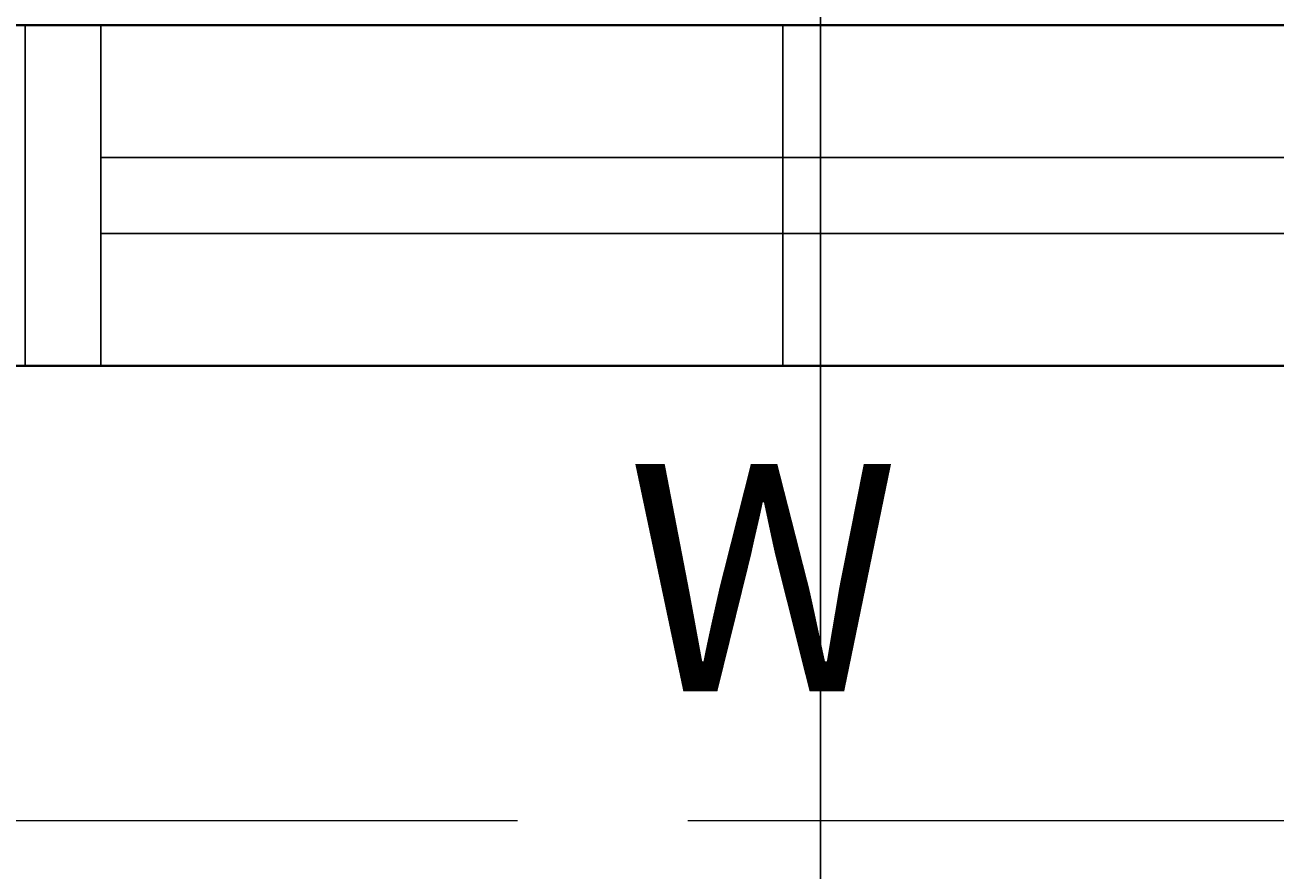
# Model space of a CAD drawing. Units: inches. Extents: x -301 to 715, y -607 to 364.
# Tile 59 of 141: x -144 to -111, y -237 to -215. Entities that reach past the tile are written whole.
import ezdxf

# ---------------------------------------------------------------- set-up
doc = ezdxf.new("R2010")
doc.units = ezdxf.units.IN
doc.header["$MEASUREMENT"] = 0
doc.linetypes.add('ACAD_ISO02W100', pattern=[15, 12, -3])
for name, color, linetype, lineweight in [('A-ANNO-DIMS', 2, 'Continuous', 18), ('A-ANNO-TEXT', 4, 'Continuous', 18), ('A-GLAZ', 2, 'Continuous', 25), ('A-GLAZ-OVHD', 2, 'ACAD_ISO02W100', 18), ('A-WALL', 3, 'Continuous', 40)]:
    doc.layers.add(name, color=color, linetype=linetype, lineweight=lineweight)
doc.styles.get("Standard").update_dxf_attribs({"font": 'arial.ttf'})
doc.dimstyles.get("Standard").update_dxf_attribs({"dimtxt": 0.18, "dimasz": 0.18, "dimexe": 0.18, "dimexo": 0.0625, "dimgap": 0.09, "dimtad": 0, "dimtih": 1, "dimtoh": 1, "dimdec": 1, "dimzin": 0, "dimdsep": 46, "dimlunit": 4, "dimtxsty": 'Standard', "dimcen": 0.09, "dimclrd": 3, "dimclre": 4, "dimclrt": 6, "dimadec": 0, "dimazin": 0, "dimtfac": 1, "dimtdec": 1, "dimtofl": 0, "dimtmove": 0, "dimatfit": 3, "dimfxl": 1, "dimtfill": 2, "dimtfillclr": 51, "dimtolj": 1, "dimtzin": 0, "dimarcsym": 0})

# ---------------------------------------------------------------- blocks, each defined once
blk = doc.blocks.new('WIN-36-PLAN')
for p, q in [((0, 0), (0, 9)), ((2, 0), (2, 9)), ((20, 0), (20, 9)), ((2, 5.5), (38, 5.5)), ((2, 3.5), (38, 3.5))]:
    blk.add_line(p, q)
blk = doc.blocks.new('WIN-SHADE-50')
at = {"ltscale": 1.5}
for p, q in [((50, 12), (0, 12)), ((45, 0), (50, 0))]:
    blk.add_line(p, q, dxfattribs=at)
blk = doc.blocks.new('*D151')
at = {"layer": 'A-ANNO-DIMS', "color": 4, "lineweight": -2, "transparency": 16777216}
for p, q in [((-204.603, -223.755), (-204.603, 359.612)), ((-45.603, -214.755), (-45.603, 359.612))]:
    blk.add_line(p, q, dxfattribs=at)
at = {"layer": 'A-ANNO-DIMS', "color": 3, "lineweight": -2, "transparency": 16777216}
for p, q in [((-204.423, 359.432), (-125.494, 359.432)), ((-45.783, 359.432), (-124.713, 359.432))]:
    blk.add_line(p, q, dxfattribs=at)
at = {"layer": 'A-ANNO-DIMS', "color": 3, "transparency": 16777216}
for points in [[(-204.423, 359.462), (-204.423, 359.402), (-204.603, 359.432)], [(-45.783, 359.462), (-45.783, 359.402), (-45.603, 359.432)]]:
    blk.add_solid(points, dxfattribs=at)
at = {"layer": 'Defpoints', "color": 0, "transparency": 16777216}
for p in [(-45.603, 359.432), (-45.603, -214.818), (-204.603, -223.818)]:
    blk.add_point(p, dxfattribs=at)
at = {"layer": 'A-ANNO-DIMS', "color": 6, "transparency": 16777216, "insert": (-125.103, 359.432), "char_height": 0.18, "attachment_point": 5, "bg_fill": 1, "box_fill_scale": 1.25, "bg_fill_color": 51, "bg_fill_transparency": 0}
blk.add_mtext('\\A1;13\'-3"', dxfattribs=at)
blk = doc.blocks.new('*D158')
at = {"layer": 'A-ANNO-DIMS', "color": 4, "lineweight": -2, "transparency": 16777216}
for p, q in [((-122.603, 221.62), (-122.603, -296.865)), ((-50.603, 221.62), (-50.603, -296.865))]:
    blk.add_line(p, q, dxfattribs=at)
at = {"layer": 'A-ANNO-DIMS', "color": 3, "lineweight": -2, "transparency": 16777216}
for p, q in [((-122.423, -296.685), (-86.933, -296.685)), ((-50.783, -296.685), (-86.274, -296.685))]:
    blk.add_line(p, q, dxfattribs=at)
at = {"layer": 'A-ANNO-DIMS', "color": 3, "transparency": 16777216}
for points in [[(-122.423, -296.655), (-122.423, -296.715), (-122.603, -296.685)], [(-50.783, -296.655), (-50.783, -296.715), (-50.603, -296.685)]]:
    blk.add_solid(points, dxfattribs=at)
at = {"layer": 'Defpoints', "color": 0, "transparency": 16777216}
for p in [(-122.603, 221.682), (-50.603, 221.682), (-50.603, -296.685)]:
    blk.add_point(p, dxfattribs=at)
at = {"layer": 'A-ANNO-DIMS', "color": 6, "transparency": 16777216, "insert": (-86.603, -296.685), "char_height": 0.18, "attachment_point": 5, "bg_fill": 1, "box_fill_scale": 1.25, "bg_fill_color": 51, "bg_fill_transparency": 0}
blk.add_mtext('\\A1;6\'-0"', dxfattribs=at)

msp = doc.modelspace()

# ---------------------------------------------------------------- linework, layer by layer
at = {"layer": 'A-WALL'}
for p, q in [((-195.603, -214.818), (-45.603, -214.818)), ((-204.603, -223.818), (-45.603, -223.818))]:
    msp.add_line(p, q, dxfattribs=at)

# ---------------------------------------------------------------- block references
at = {"layer": 'A-GLAZ'}
msp.add_blockref('WIN-36-PLAN', (-143.603, -223.818), dxfattribs=at)
at = {"layer": 'A-GLAZ-OVHD', "rotation": 180}
msp.add_blockref('WIN-SHADE-50', (-98.604, -223.817), dxfattribs=at)

# ---------------------------------------------------------------- texts
at = {"layer": 'A-ANNO-TEXT'}
msp.add_text('W', height=6, dxfattribs=at).set_placement((-127.708, -232.401))

# ---------------------------------------------------------------- dimensions: what is measured, and where the dimension line sits
at = {"layer": 'A-ANNO-DIMS'}
for base, p1, p2, picture, middle in [((-45.603, 359.432), (-204.603, -223.818), (-45.603, -214.818), '*D151', (-125.103, 359.432)), ((-50.603, -296.685), (-122.603, 221.682), (-50.603, 221.682), '*D158', (-86.603, -296.685))]:
    dim = msp.add_linear_dim(base=base, p1=p1, p2=p2, dimstyle='Standard', override={"dimdec": 1, "dimlfac": 1, "dimrnd": 0, "dimzin": 1, "dimdsep": 46, "dimlunit": 4, "dimfrac": 2}, dxfattribs=at)
    dim.commit()
    dim.dimension.update_dxf_attribs({"geometry": picture, "text_midpoint": middle})

doc.saveas('drawing.dxf')
